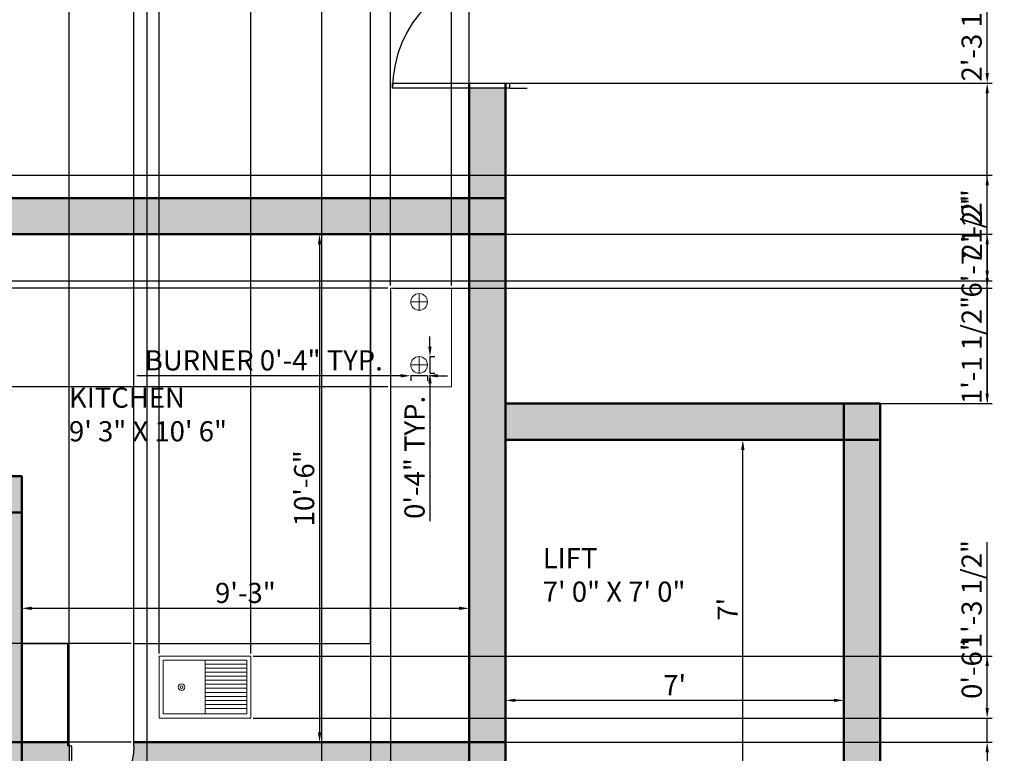
# Model space of a CAD drawing. Units: millimetres. Extents: x 2976 to 3516, y 849 to 1445.
# Tile 6 of 7: x 3272 to 3516, y 1081 to 1263. Entities that reach past the tile are written whole.
import ezdxf

# ---------------------------------------------------------------- set-up
doc = ezdxf.new("R2010")
doc.units = ezdxf.units.MM
for name, color, linetype, lineweight in [('A-AREA-IDEN', 150, 'Continuous', 25), ('A-EQPM', 130, 'Continuous', 18), ('A-FLOR-CASE', 130, 'Continuous', 25), ('A-FLOR-FIXT', 130, 'Continuous', 18), ('A-FLOR-FIXT-PATT', 130, 'Continuous', 13), ('A-WALL-PATT', 3, 'Continuous', 13), ('dimensions', 50, 'Continuous', 18), ('doors', 190, 'Continuous', 25), ('walls', 80, 'Continuous', 50)]:
    doc.layers.add(name, color=color, linetype=linetype, lineweight=lineweight)
doc.styles.get("Standard").update_dxf_attribs({"font": 'arial.ttf'})
doc.dimstyles.new('ISO-25', dxfattribs={"dimtxt": 5, "dimasz": 2.5, "dimexe": 1.25, "dimexo": 0.625, "dimtad": 1, "dimdec": 0, "dimlunit": 3, "dimtxsty": 'Standard', "dimcen": 2.5, "dimadec": 0, "dimazin": 0, "dimtfac": 1, "dimtdec": 0, "dimtmove": 0, "dimatfit": 3, "dimfxl": 1, "dimarcsym": 0})

# ---------------------------------------------------------------- blocks, each defined once
blk = doc.blocks.new('*U2')
for p, q in [((0, 0), (0, -6)), ((40, 0), (40, -6))]:
    blk.add_line(p, q)
blk.add_lwpolyline([(0, 0), (0, 40), (1.75, 40), (1.75, 0)], close=True)
blk.add_arc((0, 0), 40, 0, 90)
blk = doc.blocks.new('*D21')
at = {"layer": 'Defpoints', "color": 0, "transparency": 16777216}
for p in [(3344.23, 1209.88), (3344.23, 1083.88), (3346.57, 1083.88)]:
    blk.add_point(p, dxfattribs=at)
at = {"layer": 'dimensions', "color": 0, "lineweight": -2, "transparency": 16777216}
for p, q in [((3344.85, 1209.88), (3347.82, 1209.88)), ((3346.57, 1207.38), (3346.57, 1086.38)), ((3344.85, 1083.88), (3347.82, 1083.88))]:
    blk.add_line(p, q, dxfattribs=at)
at = {"layer": 'dimensions', "color": 0, "transparency": 16777216}
for points in [[(3346.15, 1207.38), (3346.98, 1207.38), (3346.57, 1209.88)], [(3346.15, 1086.38), (3346.98, 1086.38), (3346.57, 1083.88)]]:
    blk.add_solid(points, dxfattribs=at)
at = {"layer": 'dimensions', "color": 0, "transparency": 16777216, "insert": (3343.39, 1146.88), "char_height": 5, "attachment_point": 5, "rotation": 90}
blk.add_mtext('10\'-6"', dxfattribs=at)
blk = doc.blocks.new('*D22')
at = {"layer": 'Defpoints', "color": 0, "transparency": 16777216}
for p in [(3272.67, 1121.97), (3383.67, 1121.97), (3272.67, 1117.1)]:
    blk.add_point(p, dxfattribs=at)
at = {"layer": 'dimensions', "color": 0, "lineweight": -2, "transparency": 16777216}
for p, q in [((3272.67, 1121.34), (3272.67, 1115.85)), ((3383.67, 1121.34), (3383.67, 1115.85)), ((3381.17, 1117.1), (3275.17, 1117.1))]:
    blk.add_line(p, q, dxfattribs=at)
at = {"layer": 'dimensions', "color": 0, "transparency": 16777216}
for points in [[(3275.17, 1117.52), (3275.17, 1116.69), (3272.67, 1117.1)], [(3381.17, 1117.52), (3381.17, 1116.69), (3383.67, 1117.1)]]:
    blk.add_solid(points, dxfattribs=at)
at = {"layer": 'dimensions', "color": 0, "transparency": 16777216, "insert": (3328.17, 1120.28), "char_height": 5, "attachment_point": 5}
blk.add_mtext('9\'-3"', dxfattribs=at)
blk = doc.blocks.new('*D23')
at = {"layer": 'Defpoints', "color": 0, "transparency": 16777216}
for p in [(3392.67, 1094.28), (3392.67, 1088.66), (3476.67, 1088.66)]:
    blk.add_point(p, dxfattribs=at)
at = {"layer": 'dimensions', "color": 0, "lineweight": -2, "transparency": 16777216}
for p, q in [((3392.67, 1089.29), (3392.67, 1095.53)), ((3476.67, 1089.29), (3476.67, 1095.53)), ((3474.17, 1094.28), (3395.17, 1094.28))]:
    blk.add_line(p, q, dxfattribs=at)
at = {"layer": 'dimensions', "color": 0, "transparency": 16777216}
for points in [[(3395.17, 1094.69), (3395.17, 1093.86), (3392.67, 1094.28)], [(3474.17, 1094.69), (3474.17, 1093.86), (3476.67, 1094.28)]]:
    blk.add_solid(points, dxfattribs=at)
at = {"layer": 'dimensions', "color": 0, "transparency": 16777216, "insert": (3434.67, 1097.4), "char_height": 5, "attachment_point": 5}
blk.add_mtext("7'", dxfattribs=at)
blk = doc.blocks.new('*D24')
at = {"layer": 'Defpoints', "color": 0, "transparency": 16777216}
for p in [(3451.58, 1158.88), (3451.58, 1158.88), (3451.58, 1074.88)]:
    blk.add_point(p, dxfattribs=at)
at = {"layer": 'dimensions', "color": 0, "lineweight": -2, "transparency": 16777216}
for p, q in [((3452.2, 1158.88), (3452.83, 1158.88)), ((3451.58, 1077.38), (3451.58, 1156.38)), ((3452.2, 1074.88), (3452.83, 1074.88))]:
    blk.add_line(p, q, dxfattribs=at)
at = {"layer": 'dimensions', "color": 0, "transparency": 16777216}
for points in [[(3451.16, 1156.38), (3452, 1156.38), (3451.58, 1158.88)], [(3451.16, 1077.38), (3452, 1077.38), (3451.58, 1074.88)]]:
    blk.add_solid(points, dxfattribs=at)
at = {"layer": 'dimensions', "color": 0, "transparency": 16777216, "insert": (3448.45, 1116.88), "char_height": 5, "attachment_point": 5, "rotation": 90}
blk.add_mtext("7'", dxfattribs=at)
blk = doc.blocks.new('COOKTOP-BURNER')
for p, q in [((2.07, 4.14), (2.07, 0)), ((0, 2.07), (4.14, 2.07))]:
    blk.add_line(p, q)
blk.add_circle((2.07, 2.07), 2.07)
blk = doc.blocks.new('*D34')
at = {"layer": 'Defpoints', "color": 0, "transparency": 16777216}
for p in [(3369.2, 1175.41), (3373.34, 1175.41), (3369.2, 1174.79)]:
    blk.add_point(p, dxfattribs=at)
at = {"layer": 'dimensions', "color": 0, "lineweight": -2, "transparency": 16777216}
for p, q in [((3366.7, 1174.79), (3301.26, 1174.79)), ((3369.2, 1174.79), (3369.2, 1173.54)), ((3373.34, 1174.79), (3369.2, 1174.79)), ((3373.34, 1174.79), (3373.34, 1173.54)), ((3375.84, 1174.79), (3378.34, 1174.79))]:
    blk.add_line(p, q, dxfattribs=at)
at = {"layer": 'dimensions', "color": 0, "transparency": 16777216}
for points in [[(3366.7, 1175.21), (3366.7, 1174.38), (3369.2, 1174.79)], [(3375.84, 1175.21), (3375.84, 1174.38), (3373.34, 1174.79)]]:
    blk.add_solid(points, dxfattribs=at)
at = {"layer": 'dimensions', "color": 0, "transparency": 16777216, "insert": (3332.73, 1177.97), "char_height": 5, "attachment_point": 5}
blk.add_mtext('BURNER 0\'-4" TYP.', dxfattribs=at)
blk = doc.blocks.new('*D35')
at = {"layer": 'Defpoints', "color": 0, "transparency": 16777216}
for p in [(3373.34, 1179.55), (3373.34, 1175.41), (3373.96, 1175.41)]:
    blk.add_point(p, dxfattribs=at)
at = {"layer": 'dimensions', "color": 0, "lineweight": -2, "transparency": 16777216}
for p, q in [((3373.96, 1182.05), (3373.96, 1184.55)), ((3373.96, 1179.55), (3373.96, 1175.41)), ((3373.97, 1179.55), (3375.21, 1179.55)), ((3373.97, 1175.41), (3375.21, 1175.41)), ((3373.96, 1172.91), (3373.96, 1138.69))]:
    blk.add_line(p, q, dxfattribs=at)
at = {"layer": 'dimensions', "color": 0, "transparency": 16777216}
for points in [[(3373.54, 1182.05), (3374.38, 1182.05), (3373.96, 1179.55)], [(3373.54, 1172.91), (3374.38, 1172.91), (3373.96, 1175.41)]]:
    blk.add_solid(points, dxfattribs=at)
at = {"layer": 'dimensions', "color": 0, "transparency": 16777216, "insert": (3370.78, 1154.55), "char_height": 5, "attachment_point": 5, "rotation": 90}
blk.add_mtext('0\'-4" TYP.', dxfattribs=at)
blk = doc.blocks.new('*D55')
at = {"layer": 'Defpoints', "color": 0, "transparency": 16777216}
for p in [(3300.46, 1434.42), (3284.41, 1083.88), (3300.46, 1083.88)]:
    blk.add_point(p, dxfattribs=at)
at = {"layer": 'dimensions', "color": 0, "lineweight": -2, "transparency": 16777216}
for p, q in [((3284.41, 1084.51), (3284.41, 1435.67)), ((3286.91, 1434.42), (3297.96, 1434.42)), ((3300.46, 1084.51), (3300.46, 1435.67))]:
    blk.add_line(p, q, dxfattribs=at)
at = {"layer": 'dimensions', "color": 0, "transparency": 16777216}
for points in [[(3286.91, 1434.84), (3286.91, 1434), (3284.41, 1434.42)], [(3297.96, 1434.84), (3297.96, 1434), (3300.46, 1434.42)]]:
    blk.add_solid(points, dxfattribs=at)
at = {"layer": 'dimensions', "color": 0, "transparency": 16777216, "insert": (3292.43, 1437.56), "char_height": 5, "attachment_point": 5}
blk.add_mtext('1\'-4"', dxfattribs=at)
blk = doc.blocks.new('*D56')
at = {"layer": 'Defpoints', "color": 0, "transparency": 16777216}
for p in [(3392.67, 1275.07), (3512.21, 1275.07), (3392.67, 1247.37)]:
    blk.add_point(p, dxfattribs=at)
at = {"layer": 'dimensions', "color": 0, "lineweight": -2, "transparency": 16777216}
for p, q in [((3393.3, 1275.07), (3513.46, 1275.07)), ((3512.21, 1249.87), (3512.21, 1272.57)), ((3393.3, 1247.37), (3513.46, 1247.37))]:
    blk.add_line(p, q, dxfattribs=at)
at = {"layer": 'dimensions', "color": 0, "transparency": 16777216}
for points in [[(3511.79, 1272.57), (3512.63, 1272.57), (3512.21, 1275.07)], [(3511.79, 1249.87), (3512.63, 1249.87), (3512.21, 1247.37)]]:
    blk.add_solid(points, dxfattribs=at)
at = {"layer": 'dimensions', "color": 0, "transparency": 16777216, "insert": (3509, 1261.22), "char_height": 5, "attachment_point": 5, "rotation": 90}
blk.add_mtext('2\'-3 1/2"', dxfattribs=at)
blk = doc.blocks.new('*D59')
at = {"layer": 'Defpoints', "color": 0, "transparency": 16777216}
for p in [(3347.17, 1434.42), (3303.78, 1017.88), (3347.17, 1017.88)]:
    blk.add_point(p, dxfattribs=at)
at = {"layer": 'dimensions', "color": 0, "lineweight": -2, "transparency": 16777216}
for p, q in [((3303.78, 1018.51), (3303.78, 1435.67)), ((3306.28, 1434.42), (3344.67, 1434.42)), ((3347.17, 1018.51), (3347.17, 1435.67))]:
    blk.add_line(p, q, dxfattribs=at)
at = {"layer": 'dimensions', "color": 0, "transparency": 16777216}
for points in [[(3306.28, 1434.84), (3306.28, 1434), (3303.78, 1434.42)], [(3344.67, 1434.84), (3344.67, 1434), (3347.17, 1434.42)]]:
    blk.add_solid(points, dxfattribs=at)
at = {"layer": 'dimensions', "color": 0, "transparency": 16777216, "insert": (3325.48, 1437.63), "char_height": 5, "attachment_point": 5}
blk.add_mtext('3\'-7 1/2"', dxfattribs=at)
blk = doc.blocks.new('*D61')
at = {"layer": 'Defpoints', "color": 0, "transparency": 16777216}
for p in [(3383.67, 1434.42), (3359.24, 1209.88), (3383.67, 1209.88)]:
    blk.add_point(p, dxfattribs=at)
at = {"layer": 'dimensions', "color": 0, "lineweight": -2, "transparency": 16777216}
for p, q in [((3359.24, 1210.51), (3359.24, 1435.67)), ((3361.74, 1434.42), (3381.17, 1434.42)), ((3383.67, 1210.51), (3383.67, 1435.67)), ((3383.67, 1434.42), (3412.45, 1434.42))]:
    blk.add_line(p, q, dxfattribs=at)
at = {"layer": 'dimensions', "color": 0, "transparency": 16777216}
for points in [[(3361.74, 1434.84), (3361.74, 1434), (3359.24, 1434.42)], [(3381.17, 1434.84), (3381.17, 1434), (3383.67, 1434.42)]]:
    blk.add_solid(points, dxfattribs=at)
at = {"layer": 'dimensions', "color": 0, "transparency": 16777216, "insert": (3399.31, 1437.63), "char_height": 5, "attachment_point": 5}
blk.add_mtext('2\'-0 1/2"', dxfattribs=at)
blk = doc.blocks.new('*D62')
at = {"layer": 'Defpoints', "color": 0, "transparency": 16777216}
for p in [(3379.31, 1434.42), (3364.14, 1196.55), (3379.31, 1196.55)]:
    blk.add_point(p, dxfattribs=at)
at = {"layer": 'dimensions', "color": 0, "lineweight": -2, "transparency": 16777216}
for p, q in [((3364.14, 1197.18), (3364.14, 1435.67)), ((3366.64, 1434.42), (3376.81, 1434.42)), ((3379.31, 1197.18), (3379.31, 1435.67))]:
    blk.add_line(p, q, dxfattribs=at)
at = {"layer": 'dimensions', "color": 0, "transparency": 16777216}
for points in [[(3366.64, 1434.84), (3366.64, 1434), (3364.14, 1434.42)], [(3376.81, 1434.84), (3376.81, 1434), (3379.31, 1434.42)]]:
    blk.add_solid(points, dxfattribs=at)
at = {"layer": 'dimensions', "color": 0, "transparency": 16777216, "insert": (3371.72, 1437.6), "char_height": 5, "attachment_point": 5}
blk.add_mtext('1\'-3"', dxfattribs=at)
blk = doc.blocks.new('*D63')
at = {"layer": 'Defpoints', "color": 0, "transparency": 16777216}
for p in [(2987.13, 1196.55), (3364.14, 1196.55), (3364.14, 1172.02)]:
    blk.add_point(p, dxfattribs=at)
at = {"layer": 'dimensions', "color": 0, "lineweight": -2, "transparency": 16777216}
for p, q in [((2987.13, 1196.55), (2987.13, 1225.33)), ((3363.51, 1196.55), (2985.88, 1196.55)), ((2987.13, 1174.52), (2987.13, 1194.05)), ((3363.51, 1172.02), (2985.88, 1172.02))]:
    blk.add_line(p, q, dxfattribs=at)
at = {"layer": 'dimensions', "color": 0, "transparency": 16777216}
for points in [[(2986.71, 1194.05), (2987.55, 1194.05), (2987.13, 1196.55)], [(2986.71, 1174.52), (2987.55, 1174.52), (2987.13, 1172.02)]]:
    blk.add_solid(points, dxfattribs=at)
at = {"layer": 'dimensions', "color": 0, "transparency": 16777216, "insert": (2983.92, 1212.19), "char_height": 5, "attachment_point": 5, "rotation": 90}
blk.add_mtext('2\'-0 1/2"', dxfattribs=at)
blk = doc.blocks.new('*D64')
at = {"layer": 'Defpoints', "color": 0, "transparency": 16777216}
for p in [(3359.24, 1209.88), (3364.14, 1196.55), (3512.21, 1196.55)]:
    blk.add_point(p, dxfattribs=at)
at = {"layer": 'dimensions', "color": 0, "lineweight": -2, "transparency": 16777216}
for p, q in [((3359.87, 1209.88), (3513.46, 1209.88)), ((3512.21, 1207.38), (3512.21, 1199.05)), ((3364.76, 1196.55), (3513.46, 1196.55)), ((3512.21, 1196.55), (3512.21, 1168.33))]:
    blk.add_line(p, q, dxfattribs=at)
at = {"layer": 'dimensions', "color": 0, "transparency": 16777216}
for points in [[(3511.79, 1207.38), (3512.63, 1207.38), (3512.21, 1209.88)], [(3511.79, 1199.05), (3512.63, 1199.05), (3512.21, 1196.55)]]:
    blk.add_solid(points, dxfattribs=at)
at = {"layer": 'dimensions', "color": 0, "transparency": 16777216, "insert": (3509, 1181.19), "char_height": 5, "attachment_point": 5, "rotation": 90}
blk.add_mtext('1\'-1 1/2"', dxfattribs=at)
blk = doc.blocks.new('*D65')
at = {"layer": 'Defpoints', "color": 0, "transparency": 16777216}
for p in [(3329.5, 1434.42), (3306.79, 1105.27), (3329.5, 1105.27)]:
    blk.add_point(p, dxfattribs=at)
at = {"layer": 'dimensions', "color": 0, "lineweight": -2, "transparency": 16777216}
for p, q in [((3306.79, 1105.89), (3306.79, 1435.67)), ((3309.29, 1434.42), (3327, 1434.42)), ((3329.5, 1105.89), (3329.5, 1435.67)), ((3329.5, 1434.42), (3361.61, 1434.42))]:
    blk.add_line(p, q, dxfattribs=at)
at = {"layer": 'dimensions', "color": 0, "transparency": 16777216}
for points in [[(3309.29, 1434.84), (3309.29, 1434), (3306.79, 1434.42)], [(3327, 1434.84), (3327, 1434), (3329.5, 1434.42)]]:
    blk.add_solid(points, dxfattribs=at)
at = {"layer": 'dimensions', "color": 0, "transparency": 16777216, "insert": (3346.8, 1437.63), "char_height": 5, "attachment_point": 5}
blk.add_mtext('1\'-10 1/2"', dxfattribs=at)
blk = doc.blocks.new('*D66')
at = {"layer": 'Defpoints', "color": 0, "transparency": 16777216}
for p in [(3329.5, 1105.27), (3512.21, 1105.27), (3329.5, 1089.9)]:
    blk.add_point(p, dxfattribs=at)
at = {"layer": 'dimensions', "color": 0, "lineweight": -2, "transparency": 16777216}
for p, q in [((3512.21, 1105.27), (3512.21, 1133.49)), ((3330.12, 1105.27), (3513.46, 1105.27)), ((3512.21, 1092.4), (3512.21, 1102.77)), ((3330.12, 1089.9), (3513.46, 1089.9))]:
    blk.add_line(p, q, dxfattribs=at)
at = {"layer": 'dimensions', "color": 0, "transparency": 16777216}
for points in [[(3511.79, 1102.77), (3512.63, 1102.77), (3512.21, 1105.27)], [(3511.79, 1092.4), (3512.63, 1092.4), (3512.21, 1089.9)]]:
    blk.add_solid(points, dxfattribs=at)
at = {"layer": 'dimensions', "color": 0, "transparency": 16777216, "insert": (3509, 1120.63), "char_height": 5, "attachment_point": 5, "rotation": 90}
blk.add_mtext('1\'-3 1/2"', dxfattribs=at)
blk = doc.blocks.new('*D67')
at = {"layer": 'Defpoints', "color": 0, "transparency": 16777216}
for p in [(2987.13, 1108.35), (3300.46, 1108.35), (3300.46, 1083.88)]:
    blk.add_point(p, dxfattribs=at)
at = {"layer": 'dimensions', "color": 0, "lineweight": -2, "transparency": 16777216}
for p, q in [((2987.13, 1108.35), (2987.13, 1137.13)), ((3299.83, 1108.35), (2985.88, 1108.35)), ((2987.13, 1086.38), (2987.13, 1105.85)), ((3299.83, 1083.88), (2985.88, 1083.88))]:
    blk.add_line(p, q, dxfattribs=at)
at = {"layer": 'dimensions', "color": 0, "transparency": 16777216}
for points in [[(2986.71, 1105.85), (2987.55, 1105.85), (2987.13, 1108.35)], [(2986.71, 1086.38), (2987.55, 1086.38), (2987.13, 1083.88)]]:
    blk.add_solid(points, dxfattribs=at)
at = {"layer": 'dimensions', "color": 0, "transparency": 16777216, "insert": (2983.92, 1123.99), "char_height": 5, "attachment_point": 5, "rotation": 90}
blk.add_mtext('2\'-0 1/2"', dxfattribs=at)
blk = doc.blocks.new('*D68')
at = {"layer": 'Defpoints', "color": 0, "transparency": 16777216}
for p in [(3272.67, 1083.88), (3284.41, 1083.88), (3284.41, 853.34)]:
    blk.add_point(p, dxfattribs=at)
at = {"layer": 'dimensions', "color": 0, "lineweight": -2, "transparency": 16777216}
for p, q in [((3272.67, 1083.26), (3272.67, 852.09)), ((3284.41, 1083.26), (3284.41, 852.09)), ((3275.17, 853.34), (3281.91, 853.34)), ((3284.41, 853.34), (3316.98, 853.34))]:
    blk.add_line(p, q, dxfattribs=at)
at = {"layer": 'dimensions', "color": 0, "transparency": 16777216}
for points in [[(3275.17, 853.76), (3275.17, 852.92), (3272.67, 853.34)], [(3281.91, 853.76), (3281.91, 852.92), (3284.41, 853.34)]]:
    blk.add_solid(points, dxfattribs=at)
at = {"layer": 'dimensions', "color": 0, "transparency": 16777216, "insert": (3301.94, 856.55), "char_height": 5, "attachment_point": 5}
blk.add_mtext('0\'-11 1/2"', dxfattribs=at)
blk = doc.blocks.new('*D69')
at = {"layer": 'Defpoints', "color": 0, "transparency": 16777216}
for p in [(3306.79, 1434.42), (3300.46, 1108.35), (3306.79, 1105.27)]:
    blk.add_point(p, dxfattribs=at)
at = {"layer": 'dimensions', "color": 0, "lineweight": -2, "transparency": 16777216}
for p, q in [((3300.46, 1108.97), (3300.46, 1435.67)), ((3302.96, 1434.42), (3304.29, 1434.42)), ((3306.79, 1105.89), (3306.79, 1435.67)), ((3306.79, 1434.42), (3335.48, 1434.42))]:
    blk.add_line(p, q, dxfattribs=at)
at = {"layer": 'dimensions', "color": 0, "transparency": 16777216}
for points in [[(3302.96, 1434.84), (3302.96, 1434), (3300.46, 1434.42)], [(3304.29, 1434.84), (3304.29, 1434), (3306.79, 1434.42)]]:
    blk.add_solid(points, dxfattribs=at)
at = {"layer": 'dimensions', "color": 0, "transparency": 16777216, "insert": (3322.39, 1437.63), "char_height": 5, "attachment_point": 5}
blk.add_mtext('0\'-6 1/2"', dxfattribs=at)
blk = doc.blocks.new('*D74')
at = {"layer": 'Defpoints', "color": 0, "transparency": 16777216}
for p in [(3392.67, 1247.37), (3512.21, 1247.37), (3392.67, 1167.88)]:
    blk.add_point(p, dxfattribs=at)
at = {"layer": 'dimensions', "color": 0, "lineweight": -2, "transparency": 16777216}
for p, q in [((3393.3, 1247.37), (3513.46, 1247.37)), ((3512.21, 1170.38), (3512.21, 1244.87)), ((3393.3, 1167.88), (3513.46, 1167.88))]:
    blk.add_line(p, q, dxfattribs=at)
at = {"layer": 'dimensions', "color": 0, "transparency": 16777216}
for points in [[(3511.79, 1244.87), (3512.63, 1244.87), (3512.21, 1247.37)], [(3511.79, 1170.38), (3512.63, 1170.38), (3512.21, 1167.88)]]:
    blk.add_solid(points, dxfattribs=at)
at = {"layer": 'dimensions', "color": 0, "transparency": 16777216, "insert": (3509, 1207.63), "char_height": 5, "attachment_point": 5, "rotation": 90}
blk.add_mtext('6\'-7 1/2"', dxfattribs=at)
blk = doc.blocks.new('*D80')
at = {"layer": 'Defpoints', "color": 0, "transparency": 16777216}
for p in [(3383.67, 1434.42), (3347.17, 1017.88), (3383.67, 1008.88)]:
    blk.add_point(p, dxfattribs=at)
at = {"layer": 'dimensions', "color": 0, "lineweight": -2, "transparency": 16777216}
for p, q in [((3347.17, 1018.51), (3347.17, 1435.67)), ((3349.67, 1434.42), (3381.17, 1434.42)), ((3383.67, 1009.51), (3383.67, 1435.67))]:
    blk.add_line(p, q, dxfattribs=at)
at = {"layer": 'dimensions', "color": 0, "transparency": 16777216}
for points in [[(3349.67, 1434.84), (3349.67, 1434), (3347.17, 1434.42)], [(3381.17, 1434.84), (3381.17, 1434), (3383.67, 1434.42)]]:
    blk.add_solid(points, dxfattribs=at)
at = {"layer": 'dimensions', "color": 0, "transparency": 16777216, "insert": (3365.42, 1437.63), "char_height": 5, "attachment_point": 5}
blk.add_mtext('3\'-0 1/2"', dxfattribs=at)
blk = doc.blocks.new('*D83')
at = {"layer": 'Defpoints', "color": 0, "transparency": 16777216}
for p in [(3091.67, 1224.53), (3512.21, 1224.53), (3091.67, 1198.35)]:
    blk.add_point(p, dxfattribs=at)
at = {"layer": 'dimensions', "color": 0, "lineweight": -2, "transparency": 16777216}
for p, q in [((3092.3, 1224.53), (3513.46, 1224.53)), ((3512.21, 1200.85), (3512.21, 1222.03)), ((3092.3, 1198.35), (3513.46, 1198.35))]:
    blk.add_line(p, q, dxfattribs=at)
at = {"layer": 'dimensions', "color": 0, "transparency": 16777216}
for points in [[(3511.79, 1222.03), (3512.63, 1222.03), (3512.21, 1224.53)], [(3511.79, 1200.85), (3512.63, 1200.85), (3512.21, 1198.35)]]:
    blk.add_solid(points, dxfattribs=at)
at = {"layer": 'dimensions', "color": 0, "transparency": 16777216, "insert": (3509.08, 1211.44), "char_height": 5, "attachment_point": 5, "rotation": 90}
blk.add_mtext('2\'-2"', dxfattribs=at)
blk = doc.blocks.new('*D84')
at = {"layer": 'Defpoints', "color": 0, "transparency": 16777216}
for p in [(3359.24, 1209.88), (3364.14, 1196.55), (3364.14, 853.34)]:
    blk.add_point(p, dxfattribs=at)
at = {"layer": 'dimensions', "color": 0, "lineweight": -2, "transparency": 16777216}
for p, q in [((3359.24, 1209.26), (3359.24, 852.09)), ((3364.14, 1195.93), (3364.14, 852.09)), ((3356.74, 853.34), (3354.24, 853.34)), ((3359.24, 853.34), (3364.14, 853.34)), ((3366.64, 853.34), (3383.68, 853.34))]:
    blk.add_line(p, q, dxfattribs=at)
at = {"layer": 'dimensions', "color": 0, "transparency": 16777216}
for points in [[(3356.74, 853.76), (3356.74, 852.92), (3359.24, 853.34)], [(3366.64, 853.76), (3366.64, 852.92), (3364.14, 853.34)]]:
    blk.add_solid(points, dxfattribs=at)
at = {"layer": 'dimensions', "color": 0, "transparency": 16777216, "insert": (3376.41, 856.52), "char_height": 5, "attachment_point": 5}
blk.add_mtext('0\'-5"', dxfattribs=at)
blk = doc.blocks.new('*D85')
at = {"layer": 'Defpoints', "color": 0, "transparency": 16777216}
for p in [(3329.5, 1089.9), (3512.21, 1089.9), (3300.46, 1083.88)]:
    blk.add_point(p, dxfattribs=at)
at = {"layer": 'dimensions', "color": 0, "lineweight": -2, "transparency": 16777216}
for p, q in [((3512.21, 1092.4), (3512.21, 1109.44)), ((3330.12, 1089.9), (3513.46, 1089.9)), ((3512.21, 1083.88), (3512.21, 1089.9)), ((3301.08, 1083.88), (3513.46, 1083.88)), ((3512.21, 1081.38), (3512.21, 1078.88))]:
    blk.add_line(p, q, dxfattribs=at)
at = {"layer": 'dimensions', "color": 0, "transparency": 16777216}
for points in [[(3511.79, 1092.4), (3512.63, 1092.4), (3512.21, 1089.9)], [(3511.79, 1081.38), (3512.63, 1081.38), (3512.21, 1083.88)]]:
    blk.add_solid(points, dxfattribs=at)
at = {"layer": 'dimensions', "color": 0, "transparency": 16777216, "insert": (3509.03, 1102.17), "char_height": 5, "attachment_point": 5, "rotation": 90}
blk.add_mtext('0\'-6"', dxfattribs=at)

msp = doc.modelspace()

# ---------------------------------------------------------------- hatches: boundary and pattern name
at = {"layer": 'A-FLOR-FIXT-PATT'}
h = msp.add_hatch(dxfattribs=at)
h.set_pattern_fill('ANSI31', color=256, scale=0.3150374, angle=-45, style=0)
h.paths.add_polyline_path([(3318.15, 1092.26), (3328.5, 1092.26), (3328.5, 1104.27), (3318.15, 1104.27)])
at = {"layer": 'A-WALL-PATT'}
h = msp.add_hatch(color=256, dxfattribs=at)
h.dxf.hatch_style = 1
h.paths.add_polyline_path([(3022.67, 1398.88), (3013.67, 1398.88), (3013.67, 1278.88), (3022.67, 1278.88)])
h.paths.add_polyline_path([(3082.67, 1278.88), (3022.67, 1278.88), (3022.67, 1269.88), (3082.67, 1269.88)])
h.paths.add_polyline_path([(3022.67, 1278.88), (3013.67, 1278.88), (3013.67, 1269.88), (3022.67, 1269.88)])
h.paths.add_polyline_path([(3091.67, 1278.88), (3082.67, 1278.88), (3082.67, 1269.88), (3091.67, 1269.88)])
h.paths.add_polyline_path([(3121.76, 1278.88), (3091.67, 1278.88), (3091.67, 1269.88), (3121.76, 1269.88), (3121.76, 1272.56)])
h.paths.add_polyline_path([(3022.67, 1269.88), (3013.67, 1269.88), (3013.67, 1149.88), (3022.67, 1149.88)])
h.paths.add_polyline_path([(3022.67, 1140.88), (3013.67, 1140.88), (3013.67, 1017.88), (3022.67, 1017.88)])
h.paths.add_polyline_path([(3022.67, 1149.88), (3013.67, 1149.88), (3013.67, 1140.88), (3022.67, 1140.88)])
h.paths.add_polyline_path([(3082.67, 1149.88), (3022.67, 1149.88), (3022.67, 1140.88), (3082.67, 1140.88)])
h.paths.add_polyline_path([(3091.67, 1149.88), (3082.67, 1149.88), (3082.67, 1140.88), (3091.67, 1140.88)])
h.paths.add_polyline_path([(3143.42, 1147.68), (3143.42, 1149.88), (3091.67, 1149.88), (3091.67, 1140.88), (3144.23, 1140.88, -0.059251)])
h.paths.add_polyline_path([(3193.67, 1149.88), (3172.4, 1149.88), (3172.4, 1147.68), (3172.4, 1140.88), (3193.67, 1140.88)])
h.paths.add_polyline_path([(3202.67, 1149.88), (3193.67, 1149.88), (3193.67, 1140.88), (3202.67, 1140.88)])
h.paths.add_polyline_path([(3272.67, 1149.88), (3262.67, 1149.88), (3262.67, 1140.88), (3272.67, 1140.88)])
h.paths.add_polyline_path([(3272.67, 1140.88), (3262.67, 1140.88), (3262.67, 1083.88), (3272.67, 1083.88)])
h.paths.add_polyline_path([(3202.67, 1140.88), (3193.67, 1140.88), (3193.67, 1090.58), (3195.4, 1090.58, -0.118064), (3202.67, 1088.84)])
h.paths.add_polyline_path([(3202.67, 1074.53), (3195.4, 1074.53), (3193.67, 1074.53), (3193.67, 1017.88), (3202.67, 1017.88)])
h.paths.add_polyline_path([(3202.67, 1017.88), (3193.67, 1017.88), (3193.67, 1008.88), (3202.67, 1008.88)])
h.paths.add_polyline_path([(3193.67, 1017.88), (3112.23, 1017.88), (3112.23, 1008.88), (3193.67, 1008.88)])
h.paths.add_polyline_path([(3068.25, 1017.88), (3022.67, 1017.88), (3022.67, 1008.88), (3068.25, 1008.88)])
h.paths.add_polyline_path([(3022.67, 1017.88), (3013.67, 1017.88), (3013.67, 1008.88), (3022.67, 1008.88)])
h.paths.add_polyline_path([(3272.67, 1074.88), (3262.67, 1074.88), (3262.67, 1017.88), (3271.67, 1017.88), (3272.67, 1017.88)])
h.paths.add_polyline_path([(3272.67, 1083.88), (3262.67, 1083.88), (3262.67, 1074.88), (3272.67, 1074.88)])
h.paths.add_polyline_path([(3284.41, 1082.91), (3284.41, 1083.88), (3272.67, 1083.88), (3272.67, 1074.88), (3284.41, 1074.88)])
h.paths.add_polyline_path([(3383.67, 1083.88), (3300.46, 1083.88), (3300.46, 1082.91, -0.131652), (3298.31, 1074.88), (3383.67, 1074.88)])
h.paths.add_polyline_path([(3392.67, 1083.88), (3383.67, 1083.88), (3383.67, 1074.88), (3392.67, 1074.88)])
h.paths.add_polyline_path([(3392.67, 1074.88), (3383.67, 1074.88), (3383.67, 1017.88), (3392.67, 1017.88)])
h.paths.add_polyline_path([(3392.67, 1017.88), (3383.67, 1017.88), (3383.67, 1008.88), (3392.67, 1008.88)])
h.paths.add_polyline_path([(3383.67, 1017.88), (3347.17, 1017.88), (3347.17, 1008.88), (3383.67, 1008.88)])
h.paths.add_polyline_path([(3303.78, 1017.88), (3272.67, 1017.88), (3272.67, 1008.88), (3303.78, 1008.88)])
h.paths.add_polyline_path([(3272.67, 1017.88), (3271.67, 1017.88), (3262.67, 1017.88), (3262.67, 1008.88), (3272.67, 1008.88)])
h.paths.add_polyline_path([(3262.67, 1017.88), (3243.44, 1017.88), (3243.44, 1008.88), (3262.67, 1008.88)])
h.paths.add_polyline_path([(3218.58, 1017.88), (3202.67, 1017.88), (3202.67, 1008.88), (3218.58, 1008.88)])
h.paths.add_polyline_path([(3392.67, 1209.88), (3383.67, 1209.88), (3383.67, 1083.88), (3392.67, 1083.88)])
h.paths.add_polyline_path([(3392.67, 1218.88), (3383.67, 1218.88), (3383.67, 1209.88), (3392.67, 1209.88)])
h.paths.add_polyline_path([(3392.67, 1246.1), (3383.67, 1246.1), (3383.67, 1218.88), (3392.67, 1218.88)])
h.paths.add_polyline_path([(3383.67, 1218.88), (3251.67, 1218.88), (3251.67, 1209.88), (3383.67, 1209.88)])
h.paths.add_polyline_path([(3251.67, 1287.88), (3242.67, 1287.88), (3242.67, 1218.88), (3251.67, 1218.88)])
h.paths.add_polyline_path([(3251.67, 1218.88), (3242.67, 1218.88), (3242.67, 1209.88), (3251.67, 1209.88)])
h.paths.add_polyline_path([(3251.67, 1398.88), (3242.67, 1398.88), (3242.67, 1296.88), (3251.67, 1296.88)])
h.paths.add_polyline_path([(3251.67, 1296.88), (3242.67, 1296.88), (3242.67, 1287.88), (3251.67, 1287.88)])
h.paths.add_polyline_path([(3242.67, 1296.88), (3182.67, 1296.88), (3182.67, 1287.88), (3242.67, 1287.88)])
h.paths.add_polyline_path([(3182.67, 1296.88), (3173.67, 1296.88), (3173.67, 1287.88), (3182.67, 1287.88)])
h.paths.add_polyline_path([(3182.67, 1287.88), (3173.67, 1287.88), (3173.67, 1278.88), (3182.67, 1278.88)])
h.paths.add_polyline_path([(3182.67, 1278.88), (3173.67, 1278.88), (3173.67, 1269.88), (3182.67, 1269.88)])
h.paths.add_polyline_path([(3173.67, 1278.88), (3150.05, 1278.88, -0.054989), (3150.74, 1272.56), (3150.74, 1269.88), (3173.67, 1269.88)])
h.paths.add_polyline_path([(3182.67, 1398.88), (3173.67, 1398.88), (3173.67, 1296.88), (3182.67, 1296.88)])
h.paths.add_polyline_path([(3182.67, 1407.88), (3173.67, 1407.88), (3173.67, 1398.88), (3182.67, 1398.88)])
h.paths.add_polyline_path([(3173.67, 1407.88), (3104.59, 1407.88), (3104.59, 1398.88), (3173.67, 1398.88)])
h.paths.add_polyline_path([(3060.33, 1407.88), (3022.67, 1407.88), (3022.67, 1398.88), (3060.33, 1398.88)])
h.paths.add_polyline_path([(3022.67, 1407.88), (3013.67, 1407.88), (3013.67, 1398.88), (3022.67, 1398.88)])
h.paths.add_polyline_path([(3196.7, 1407.88), (3182.67, 1407.88), (3182.67, 1398.88), (3196.7, 1398.88)])
h.paths.add_polyline_path([(3242.67, 1407.88), (3223.57, 1407.88), (3223.57, 1398.88), (3242.67, 1398.88)])
h.paths.add_polyline_path([(3251.67, 1407.88), (3242.67, 1407.88), (3242.67, 1398.88), (3251.67, 1398.88)])
h.paths.add_polyline_path([(3295.02, 1407.88), (3251.67, 1407.88), (3251.67, 1398.88), (3295.02, 1398.88)])
h.paths.add_polyline_path([(3383.67, 1407.88), (3338.5, 1407.88), (3338.5, 1398.88), (3383.67, 1398.88)])
h.paths.add_polyline_path([(3392.67, 1407.88), (3383.67, 1407.88), (3383.67, 1398.88), (3392.67, 1398.88)])
h.paths.add_polyline_path([(3392.67, 1398.88), (3383.67, 1398.88), (3383.67, 1273.3, -0.079613), (3392.67, 1275.07)])
h = msp.add_hatch(color=256, dxfattribs=at)
h.dxf.hatch_style = 1
h.paths.add_polyline_path([(3476.67, 1167.88), (3392.67, 1167.88), (3392.67, 1158.88), (3476.67, 1158.88)])
h.paths.add_polyline_path([(3485.67, 1167.88), (3476.67, 1167.88), (3476.67, 1158.88), (3485.67, 1158.88)])
h.paths.add_polyline_path([(3485.67, 1074.88), (3476.67, 1074.88), (3476.67, 1065.88), (3485.67, 1065.88)])
h.paths.add_polyline_path([(3485.67, 1065.88), (3476.67, 1065.88), (3476.67, 981.88), (3485.67, 981.88)])
h.paths.add_polyline_path([(3485.67, 1158.88), (3476.67, 1158.88), (3476.67, 1074.88), (3485.67, 1074.88)])
h.paths.add_polyline_path([(3476.67, 1074.88), (3392.67, 1074.88), (3392.67, 1065.88), (3476.67, 1065.88)])
h.paths.add_polyline_path([(3476.67, 981.88), (3392.67, 981.88), (3392.67, 972.88), (3476.67, 972.88)])
h.paths.add_polyline_path([(3485.67, 972.88), (3476.67, 972.88), (3476.67, 888.88), (3485.67, 888.88)])
h.paths.add_polyline_path([(3485.67, 981.88), (3476.67, 981.88), (3476.67, 972.88), (3485.67, 972.88)])
h.paths.add_polyline_path([(3476.67, 888.88), (3392.67, 888.88), (3392.67, 879.88), (3476.67, 879.88)])
h.paths.add_polyline_path([(3485.67, 888.88), (3476.67, 888.88), (3476.67, 879.88), (3485.67, 879.88)])

# ---------------------------------------------------------------- linework, layer by layer
at = {"layer": 'A-EQPM'}
msp.add_lwpolyline([(3364.14, 1196.55), (3379.31, 1196.55), (3379.31, 1172.02), (3364.14, 1172.02)], close=True, dxfattribs=at)
at = {"layer": 'A-FLOR-CASE'}
for p, q in [((3359.24, 1108.35), (3359.24, 1209.88)), ((3359.24, 1209.88), (3359.24, 1108.35)), ((3272.67, 1083.88), (3272.67, 1108.35)), ((3272.67, 1108.35), (3284.07, 1108.35)), ((3284.07, 1108.35), (3284.07, 1082.91)), ((3300.46, 1083.88), (3300.46, 1108.35)), ((3300.46, 1108.35), (3359.24, 1108.35)), ((3359.24, 1083.88), (3300.46, 1083.88))]:
    msp.add_line(p, q, dxfattribs=at)
at = {"layer": 'A-FLOR-FIXT'}
msp.add_line((3318.15, 1104.27), (3318.15, 1090.9), dxfattribs=at)
for points in [[(3306.79, 1105.27), (3329.5, 1105.27), (3329.5, 1089.9), (3306.79, 1089.9)], [(3307.79, 1104.27), (3328.5, 1104.27), (3328.5, 1090.9), (3307.79, 1090.9)]]:
    msp.add_lwpolyline(points, close=True, dxfattribs=at)
for radius in [0.812, 0.351]:
    msp.add_circle((3312.3, 1097.55), radius, dxfattribs=at)
at = {"layer": 'walls'}
for p, q in [((3383.67, 1247.37), (3383.67, 1209.88)), ((3392.67, 1247.37), (3392.67, 1209.88)), ((3242.67, 1218.88), (3392.67, 1218.88)), ((3242.67, 1209.88), (3392.67, 1209.88)), ((3383.67, 1209.88), (3383.67, 1008.88)), ((3392.67, 1209.88), (3392.67, 1008.88)), ((3392.67, 1167.88), (3485.67, 1167.88)), ((3476.67, 879.88), (3476.67, 1167.88)), ((3485.67, 879.88), (3485.67, 1167.88)), ((3392.67, 1158.88), (3485.67, 1158.88)), ((3262.67, 1149.88), (3272.67, 1149.88)), ((3272.67, 1149.88), (3272.67, 1008.88)), ((3262.67, 1140.88), (3272.67, 1140.88)), ((3262.67, 1083.88), (3284.41, 1083.88)), ((3300.46, 1083.88), (3392.67, 1083.88))]:
    msp.add_line(p, q, dxfattribs=at)

# ---------------------------------------------------------------- block references
at = {"layer": 'A-EQPM'}
msp.add_blockref('COOKTOP-BURNER', (3369.2, 1191.04), dxfattribs=at)
at = {"layer": 'A-EQPM', "rotation": 180}
msp.add_blockref('COOKTOP-BURNER', (3373.34, 1179.55), dxfattribs=at)
at = {"layer": 'doors'}
for p, xscale, yscale, zscale, rotation in [((3393.69, 1246.1), 0.7246062005204927, 0.7246062005204927, 0.7246062005204927, 90), ((3284.41, 1082.91), -0.4013541687362427, 0.4013541687362427, 0.4013541687362427, 180)]:
    msp.add_blockref('*U2', p, dxfattribs=dict(at, xscale=xscale, yscale=yscale, zscale=zscale, rotation=rotation))

# ---------------------------------------------------------------- texts
at = {"layer": 'A-AREA-IDEN', "char_height": 5, "attachment_point": 1}
for s, width, insert in [('KITCHEN\\P9\' 3" X 10\' 6"', 51.1718, (3284.4, 1171.86)), ('LIFT \\P7\' 0" X 7\' 0"', 61.837, (3401.94, 1132.06))]:
    msp.add_mtext_dynamic_manual_height_columns(s, width=width, gutter_width=12.5, heights=[0], dxfattribs=dict(at, insert=insert))

# ---------------------------------------------------------------- dimensions: what is measured, and where the dimension line sits
at = {"layer": 'dimensions'}
for base, p1, p2, override, picture, middle in [((3306.79, 1434.42), (3300.46, 1108.35), (3306.79, 1105.27), {"dimdec": 1, "dimlfac": 1, "dimrnd": 0, "dimzin": 1, "dimdsep": 46, "dimlunit": 4, "dimfrac": 2}, '*D69', (3322.39, 1437.63)), ((3347.17, 1434.42), (3303.78, 1017.88), (3347.17, 1017.88), {"dimdec": 1, "dimlfac": 1, "dimrnd": 0, "dimzin": 1, "dimdsep": 46, "dimlunit": 4, "dimfrac": 2}, '*D59', (3325.48, 1437.63)), ((3329.5, 1434.42), (3306.79, 1105.27), (3329.5, 1105.27), {"dimdec": 1, "dimlfac": 1, "dimrnd": 0, "dimzin": 1, "dimdsep": 46, "dimlunit": 4, "dimfrac": 2}, '*D65', (3346.8, 1437.63)), ((3383.67, 1434.42), (3347.17, 1017.88), (3383.67, 1008.88), {"dimdec": 1, "dimlfac": 1, "dimrnd": 0, "dimzin": 1, "dimdsep": 46, "dimlunit": 4, "dimfrac": 2}, '*D80', (3365.42, 1437.63)), ((3383.67, 1434.42), (3359.24, 1209.88), (3383.67, 1209.88), {"dimdec": 1, "dimlfac": 1, "dimrnd": 0, "dimzin": 1, "dimdsep": 46, "dimlunit": 4, "dimfrac": 2}, '*D61', (3399.31, 1437.63)), ((3300.4593, 1434.4215), (3284.4052, 1083.8815), (3300.4593, 1083.8815), {"dimdec": 1, "dimlfac": 1, "dimrnd": 0, "dimzin": 1, "dimdsep": 46, "dimlunit": 4, "dimfrac": 2}, '*D55', (3292.4322, 1437.5567)), ((3379.31, 1434.42), (3364.14, 1196.55), (3379.31, 1196.55), {"dimdec": 1, "dimlfac": 1, "dimrnd": 0, "dimzin": 1, "dimdsep": 46, "dimlunit": 4, "dimfrac": 2}, '*D62', (3371.72, 1437.6)), ((3364.14, 853.34), (3359.24, 1209.88), (3364.14, 1196.55), {"dimdec": 1, "dimlfac": 1, "dimrnd": 0, "dimzin": 1, "dimdsep": 46, "dimlunit": 4, "dimfrac": 2}, '*D84', (3376.41, 856.52)), ((3272.67, 1117.1), (3383.67, 1121.97), (3272.67, 1121.97), {"dimclrd": 0, "dimclre": 0, "dimclrt": 0}, '*D22', (3328.17, 1120.28)), ((3392.67, 1094.28), (3476.67, 1088.66), (3392.67, 1088.66), {"dimclrd": 0, "dimclre": 0, "dimclrt": 0}, '*D23', (3434.67, 1097.4)), ((3284.41, 853.34), (3272.67, 1083.88), (3284.41, 1083.88), {"dimdec": 1, "dimlfac": 1, "dimrnd": 0, "dimzin": 1, "dimdsep": 46, "dimlunit": 4, "dimfrac": 2}, '*D68', (3301.94, 856.55))]:
    dim = msp.add_linear_dim(base=base, p1=p1, p2=p2, dimstyle='ISO-25', override=override, dxfattribs=at)
    dim.commit()
    dim.dimension.update_dxf_attribs({"geometry": picture, "text_midpoint": middle})
for base, p1, p2, override, picture, middle in [((3512.21, 1275.07), (3392.67, 1247.37), (3392.67, 1275.07), {"dimdec": 1, "dimlfac": 1, "dimrnd": 0, "dimzin": 1, "dimdsep": 46, "dimlunit": 4, "dimfrac": 2}, '*D56', (3509, 1261.22)), ((3512.21, 1247.37), (3392.67, 1167.88), (3392.67, 1247.37), {"dimdec": 1, "dimlfac": 1, "dimrnd": 0, "dimzin": 1, "dimdsep": 46, "dimlunit": 4, "dimfrac": 2}, '*D74', (3509, 1207.63)), ((2987.13, 1196.55), (3364.14, 1172.02), (3364.14, 1196.55), {"dimdec": 1, "dimlfac": 1, "dimrnd": 0, "dimzin": 1, "dimdsep": 46, "dimlunit": 4, "dimfrac": 2}, '*D63', (2983.92, 1212.19)), ((3512.21, 1224.53), (3091.67, 1198.35), (3091.67, 1224.53), {"dimdec": 1, "dimlfac": 1, "dimrnd": 0, "dimzin": 1, "dimdsep": 46, "dimlunit": 4, "dimfrac": 2}, '*D83', (3509.08, 1211.44)), ((3346.57, 1083.88), (3344.23, 1209.88), (3344.23, 1083.88), {"dimclrd": 0, "dimclre": 0, "dimclrt": 0}, '*D21', (3343.39, 1146.88)), ((3512.21, 1196.55), (3359.24, 1209.88), (3364.14, 1196.55), {"dimdec": 1, "dimlfac": 1, "dimrnd": 0, "dimzin": 1, "dimdsep": 46, "dimlunit": 4, "dimfrac": 2}, '*D64', (3509, 1181.19)), ((3451.58, 1158.88), (3451.58, 1074.88), (3451.58, 1158.88), {"dimclrd": 0, "dimclre": 0, "dimclrt": 0}, '*D24', (3448.45, 1116.88)), ((2987.13, 1108.35), (3300.46, 1083.88), (3300.46, 1108.35), {"dimdec": 1, "dimlfac": 1, "dimrnd": 0, "dimzin": 1, "dimdsep": 46, "dimlunit": 4, "dimfrac": 2}, '*D67', (2983.92, 1123.99)), ((3512.21, 1105.27), (3329.5, 1089.9), (3329.5, 1105.27), {"dimdec": 1, "dimlfac": 1, "dimrnd": 0, "dimzin": 1, "dimdsep": 46, "dimlunit": 4, "dimfrac": 2}, '*D66', (3509, 1120.63)), ((3512.21, 1089.9), (3300.46, 1083.88), (3329.5, 1089.9), {"dimdec": 1, "dimlfac": 1, "dimrnd": 0, "dimzin": 1, "dimdsep": 46, "dimlunit": 4, "dimfrac": 2}, '*D85', (3509.03, 1102.17))]:
    dim = msp.add_linear_dim(base=base, p1=p1, p2=p2, angle=90, dimstyle='ISO-25', override=override, dxfattribs=at)
    dim.commit()
    dim.dimension.update_dxf_attribs({"geometry": picture, "text_midpoint": middle})
for base, p1, p2, angle, text, picture, middle in [((3369.2, 1174.79), (3373.34, 1175.41), (3369.2, 1175.41), 180, 'BURNER <> TYP.', '*D34', (3332.73, 1177.97)), ((3373.96, 1175.41), (3373.34, 1179.55), (3373.34, 1175.41), 270, '<> TYP.', '*D35', (3370.78, 1154.55))]:
    dim = msp.add_linear_dim(base=base, p1=p1, p2=p2, angle=angle, text=text, dimstyle='ISO-25', override={"dimdec": 1, "dimlfac": 1, "dimrnd": 0, "dimzin": 1, "dimdsep": 46, "dimlunit": 4, "dimfrac": 2}, dxfattribs=at)
    dim.commit()
    dim.dimension.update_dxf_attribs({"geometry": picture, "text_midpoint": middle})

doc.saveas('drawing.dxf')
